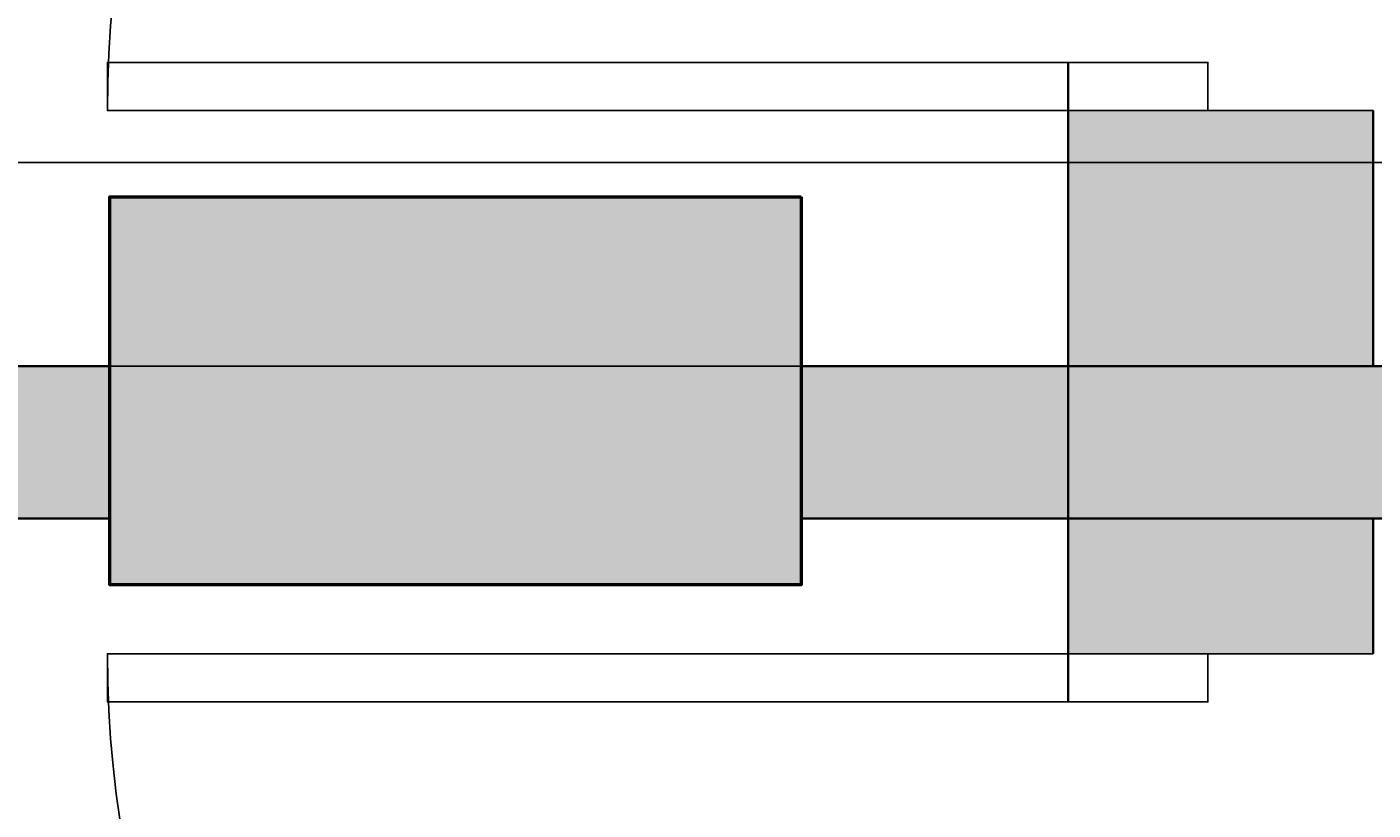
# Model space of a CAD drawing. Units: inches. Extents: x 1998 to 2588, y 1139 to 1977.
# Tile 8 of 134: x 2075 to 2115, y 1576 to 1599. Entities that reach past the tile are written whole.
import ezdxf

# ---------------------------------------------------------------- set-up
doc = ezdxf.new("R2010")
doc.units = ezdxf.units.IN
for name, color, linetype, lineweight in [('A-ANNO-DIMS', 2, 'Continuous', 18), ('A-COLS-PATT', 250, 'Continuous', 13), ('A-WALL-PATT', 252, 'Continuous', 13), ('COLUMN', 10, 'Continuous', 50), ('DOOR', 52, 'Continuous', 25), ('WALL', 200, 'Continuous', 35)]:
    doc.layers.add(name, color=color, linetype=linetype, lineweight=lineweight)
doc.styles.get("Standard").update_dxf_attribs({"font": 'arial.ttf'})
doc.dimstyles.get("Standard").update_dxf_attribs({"dimtxt": 0.18, "dimasz": 0.18, "dimexe": 0.18, "dimexo": 0.0625, "dimgap": 0.09, "dimtad": 0, "dimtih": 1, "dimtoh": 1, "dimdec": 4, "dimzin": 0, "dimdsep": 46, "dimtxsty": 'Standard', "dimcen": 0.09, "dimadec": 0, "dimazin": 0, "dimtfac": 1, "dimtdec": 4, "dimtofl": 0, "dimtmove": 0, "dimatfit": 3, "dimfxl": 1, "dimtolj": 1, "dimtzin": 0, "dimarcsym": 0})

# ---------------------------------------------------------------- blocks, each defined once
blk = doc.blocks.new('*U2')
for p, q in [((0, 0), (0, -6)), ((40, 0), (40, -6))]:
    blk.add_line(p, q)
blk.add_lwpolyline([(0, 0), (0, 40), (1.75, 40), (1.75, 0)], close=True)
blk.add_arc((0, 0), 40, 0, 90)
blk = doc.blocks.new('*D30')
at = {"layer": 'A-ANNO-DIMS', "color": 0, "lineweight": -2, "transparency": 16777216}
for p, q in [((2407.91, 1636.732), (1997.843, 1636.732)), ((1998.023, 1636.552), (1998.023, 1615.913)), ((1998.023, 1594.912), (1998.023, 1615.552)), ((2407.91, 1594.732), (1997.843, 1594.732))]:
    blk.add_line(p, q, dxfattribs=at)
at = {"layer": 'A-ANNO-DIMS', "color": 0, "transparency": 16777216}
for points in [[(1997.993, 1636.552), (1998.053, 1636.552), (1998.023, 1636.732)], [(1997.993, 1594.912), (1998.053, 1594.912), (1998.023, 1594.732)]]:
    blk.add_solid(points, dxfattribs=at)
at = {"layer": 'Defpoints', "color": 0, "transparency": 16777216}
for p in [(1998.023, 1636.732), (2407.973, 1636.732), (2407.973, 1594.732)]:
    blk.add_point(p, dxfattribs=at)
at = {"layer": 'A-ANNO-DIMS', "color": 0, "transparency": 16777216, "insert": (1998.023, 1615.732), "char_height": 0.18, "attachment_point": 5}
blk.add_mtext('\\A1;42', dxfattribs=at)
blk = doc.blocks.new('*D34')
at = {"layer": 'A-ANNO-DIMS', "color": 0, "lineweight": -2, "transparency": 16777216}
for p, q in [((2407.91, 1594.732), (1997.843, 1594.732)), ((1998.023, 1594.552), (1998.023, 1558.913)), ((1998.023, 1522.912), (1998.023, 1558.552)), ((2407.91, 1522.732), (1997.843, 1522.732))]:
    blk.add_line(p, q, dxfattribs=at)
at = {"layer": 'A-ANNO-DIMS', "color": 0, "transparency": 16777216}
for points in [[(1997.993, 1594.552), (1998.053, 1594.552), (1998.023, 1594.732)], [(1997.993, 1522.912), (1998.053, 1522.912), (1998.023, 1522.732)]]:
    blk.add_solid(points, dxfattribs=at)
at = {"layer": 'Defpoints', "color": 0, "transparency": 16777216}
for p in [(1998.023, 1594.732), (2407.973, 1594.732), (2407.973, 1522.732)]:
    blk.add_point(p, dxfattribs=at)
at = {"layer": 'A-ANNO-DIMS', "color": 0, "transparency": 16777216, "insert": (1998.023, 1558.732), "char_height": 0.18, "attachment_point": 5}
blk.add_mtext('\\A1;72', dxfattribs=at)
blk = doc.blocks.new('*D35')
at = {"layer": 'A-ANNO-DIMS', "color": 0, "lineweight": -2, "transparency": 16777216}
for p, q in [((2148.392, 1612.732), (1997.843, 1612.732)), ((1998.023, 1612.552), (1998.023, 1600.913)), ((1998.023, 1588.912), (1998.023, 1600.552)), ((2148.392, 1588.732), (1997.843, 1588.732))]:
    blk.add_line(p, q, dxfattribs=at)
at = {"layer": 'A-ANNO-DIMS', "color": 0, "transparency": 16777216}
for points in [[(1997.993, 1612.552), (1998.053, 1612.552), (1998.023, 1612.732)], [(1997.993, 1588.912), (1998.053, 1588.912), (1998.023, 1588.732)]]:
    blk.add_solid(points, dxfattribs=at)
at = {"layer": 'Defpoints', "color": 0, "transparency": 16777216}
for p in [(1998.023, 1612.732), (2148.455, 1612.732), (2148.455, 1588.732)]:
    blk.add_point(p, dxfattribs=at)
at = {"layer": 'A-ANNO-DIMS', "color": 0, "transparency": 16777216, "insert": (1998.023, 1600.732), "char_height": 0.18, "attachment_point": 5}
blk.add_mtext('\\A1;24', dxfattribs=at)

msp = doc.modelspace()

# ---------------------------------------------------------------- hatches: boundary and pattern name
at = {"layer": 'A-COLS-PATT'}
h = msp.add_hatch(color=256, dxfattribs=at)
h.dxf.hatch_style = 1
h.paths.add_polyline_path([(2099.4125, 1888.7324), (2087.9729, 1888.7324), (2087.9729, 1868.3278), (2099.4125, 1868.3278)])
h.paths.add_polyline_path([(2234.4125, 1888.7324), (2222.9729, 1888.7324), (2222.9729, 1868.3278), (2234.4125, 1868.3278)])
h.paths.add_polyline_path([(2341.4729, 1886.637), (2330.0332, 1886.637), (2330.0332, 1866.2324), (2341.4729, 1866.2324)])
h.paths.add_polyline_path([(2507.8006, 1882.7324), (2487.396, 1882.7324), (2487.396, 1871.2927), (2507.8006, 1871.2927)])
h.paths.add_polyline_path([(2510.9729, 1766.672), (2490.5682, 1766.672), (2490.5682, 1755.2324), (2510.9729, 1755.2324)])
h.paths.add_polyline_path([(2345.9729, 1759.7324), (2334.5332, 1759.7324), (2334.5332, 1739.3278), (2345.9729, 1739.3278)])
h.paths.add_polyline_path([(2234.4125, 1774.3318), (2222.9729, 1774.3318), (2222.9729, 1753.9272), (2234.4125, 1753.9272)])
h.paths.add_polyline_path([(2099.4125, 1775.637), (2087.9729, 1775.637), (2087.9729, 1755.2324), (2099.4125, 1755.2324)])
h.paths.add_polyline_path([(2098.0956, 1593.7241), (2077.691, 1593.7241), (2077.691, 1582.2845), (2098.0956, 1582.2845)])
h.paths.add_polyline_path([(2227.4729, 1604.637), (2216.0332, 1604.637), (2216.0332, 1584.2324), (2227.4729, 1584.2324)])
h.paths.add_polyline_path([(2345.9729, 1647.5211), (2334.5332, 1647.5211), (2334.5332, 1627.1165), (2345.9729, 1627.1165)])
h.paths.add_polyline_path([(2522.3775, 1641.2324), (2501.9729, 1641.2324), (2501.9729, 1629.7927), (2522.3775, 1629.7927)])
h.paths.add_polyline_path([(2522.3775, 1480.7324), (2501.9729, 1480.7324), (2501.9729, 1469.2927), (2522.3775, 1469.2927)])
h.paths.add_polyline_path([(2345.9729, 1488.5616), (2334.5332, 1488.5616), (2334.5332, 1468.1569), (2345.9729, 1468.1569)])
h.paths.add_polyline_path([(2234.4125, 1486.137), (2227.4729, 1486.137), (2227.4729, 1465.7324), (2234.4125, 1465.7324)])
h.paths.add_polyline_path([(2227.4729, 1486.137), (2222.9729, 1486.137), (2222.9729, 1465.7324), (2227.4729, 1465.7324)])
h.paths.add_polyline_path([(2108.3775, 1470.2324), (2087.9729, 1470.2324), (2087.9729, 1458.7927), (2108.3775, 1458.7927)])
h.paths.add_polyline_path([(2096.9729, 1365.5012), (2087.9729, 1365.5012), (2087.9729, 1345.0966), (2096.9729, 1345.0966)])
h.paths.add_polyline_path([(2087.9729, 1365.5012), (2085.5332, 1365.5012), (2085.5332, 1345.0966), (2087.9729, 1345.0966)])
h.paths.add_polyline_path([(2234.4125, 1285.137), (2222.9729, 1285.137), (2222.9729, 1264.7324), (2234.4125, 1264.7324)])
h.paths.add_polyline_path([(2345.9729, 1285.137), (2334.5332, 1285.137), (2334.5332, 1264.7324), (2345.9729, 1264.7324)])
h.paths.add_polyline_path([(2503.1458, 1240.172), (2482.7412, 1240.172), (2482.7412, 1228.7324), (2503.1458, 1228.7324)])
h.paths.add_polyline_path([(2510.9729, 1369.172), (2490.5682, 1369.172), (2490.5682, 1357.7324), (2510.9729, 1357.7324)])
at = {"layer": 'A-WALL-PATT'}
h = msp.add_hatch(color=256, dxfattribs=at)
h.dxf.hatch_style = 1
h.paths.add_polyline_path([(2222.9729, 1888.7324), (2099.4125, 1888.7324), (2099.4125, 1879.7324), (2222.9729, 1879.7324)])
h.paths.add_polyline_path([(2096.9729, 1868.3278), (2087.9729, 1868.3278), (2087.9729, 1775.637), (2096.9729, 1775.637)])
h.paths.add_polyline_path([(2227.4729, 1868.3278), (2222.9729, 1868.3278), (2222.9729, 1774.3318), (2227.4729, 1774.3318)])
h.paths.add_polyline_path([(2188.3019, 1759.7324), (2138.6074, 1759.7324), (2099.4125, 1759.7324), (2099.4125, 1755.2324), (2176.9729, 1755.2324), (2188.3019, 1755.2324)])
h.paths.add_polyline_path([(2087.9729, 1759.7324), (2059.4729, 1759.7324), (2059.4729, 1702.7324), (2087.9729, 1702.7324), (2087.9729, 1707.2324), (2063.9729, 1707.2324), (2063.9729, 1755.2324), (2087.9729, 1755.2324)])
h.paths.add_polyline_path([(2096.9729, 1755.2324), (2087.9729, 1755.2324), (2087.9729, 1707.2324), (2096.9729, 1707.2324)])
h.paths.add_polyline_path([(2187.0461, 1707.2324), (2105.9729, 1707.2324), (2096.9729, 1707.2324), (2087.9729, 1707.2324), (2087.9729, 1702.7324), (2105.9729, 1702.7324), (2114.9729, 1702.7324), (2187.0461, 1702.7324)])
h.paths.add_polyline_path([(2181.4729, 1719.2028), (2176.9729, 1719.2028), (2176.9729, 1707.2324), (2181.4729, 1707.2324)])
h.paths.add_polyline_path([(2216.0332, 1588.7324), (2114.9729, 1588.7324), (2105.9729, 1588.7324), (2105.9729, 1584.2324), (2216.0332, 1584.2324)])
h.paths.add_polyline_path([(2077.691, 1588.7324), (2061.4729, 1588.7324), (2061.4729, 1584.2324), (2077.691, 1584.2324)])
h.paths.add_polyline_path([(2105.9729, 1588.7324), (2098.0956, 1588.7324), (2098.0956, 1584.2324), (2105.9729, 1584.2324)])
h.paths.add_polyline_path([(2114.9729, 1596.2642), (2110.1012, 1596.2642), (2105.9729, 1596.2642), (2105.9729, 1588.7324), (2114.9729, 1588.7324)])
h.paths.add_polyline_path([(2114.9729, 1584.2324), (2105.9729, 1584.2324), (2105.9729, 1580.249), (2110.1012, 1580.249), (2114.9729, 1580.249)])
h.paths.add_polyline_path([(2114.9729, 1547.7716), (2110.1012, 1547.7716, -0.0318759), (2105.9729, 1548.035), (2105.9729, 1470.2324), (2108.3775, 1470.2324), (2108.3775, 1465.7324), (2186.2943, 1465.7324), (2186.2943, 1470.2324), (2114.9729, 1470.2324)])
h.paths.add_polyline_path([(2227.4729, 1584.2324), (2222.9729, 1584.2324), (2222.9729, 1486.137), (2227.4729, 1486.137)])
h.paths.add_polyline_path([(2295.4138, 1593.2324), (2227.4729, 1593.2324), (2227.4729, 1588.7324), (2295.4138, 1588.7324), (2295.4138, 1591.8729)])
h.paths.add_polyline_path([(2345.9729, 1627.1165), (2341.4729, 1627.1165), (2341.4729, 1593.2324), (2337.2869, 1593.2324), (2337.2869, 1591.8729), (2337.2869, 1588.7324), (2345.9729, 1588.7324)])
h.paths.add_polyline_path([(2291.9729, 1588.7324), (2287.4729, 1588.7324), (2287.4729, 1522.7324), (2291.9729, 1522.7324)])
h.paths.add_polyline_path([(2291.9729, 1522.7324), (2287.4729, 1522.7324), (2227.4729, 1522.7324), (2227.4729, 1518.2324), (2291.9729, 1518.2324)])
h.paths.add_polyline_path([(2295.7347, 1519.5919), (2295.7347, 1522.7324), (2291.9729, 1522.7324), (2291.9729, 1518.2324), (2295.7347, 1518.2324)])
h.paths.add_polyline_path([(2345.9729, 1522.7324), (2337.6078, 1522.7324), (2337.6078, 1519.5919), (2337.6078, 1518.2324), (2341.4729, 1518.2324), (2341.4729, 1488.5616), (2345.9729, 1488.5616)])
h.paths.add_polyline_path([(2345.9729, 1468.1569), (2341.4729, 1468.1569), (2341.4729, 1374.2324), (2227.4729, 1374.2324), (2227.4729, 1369.7324), (2345.9729, 1369.7324)])
h.paths.add_polyline_path([(2345.9729, 1369.7324), (2341.4729, 1369.7324), (2341.4729, 1362.2324), (2345.9729, 1362.2324)])
h.paths.add_polyline_path([(2345.9729, 1317.7324), (2345.9729, 1322.2324), (2341.4729, 1322.2324), (2341.4729, 1285.137), (2345.9729, 1285.137)], flags=17)
h.paths.add_polyline_path([(2356.2096, 1322.2324), (2345.9729, 1322.2324), (2345.9729, 1317.7324), (2356.2096, 1317.7324), (2356.2096, 1319.3088)], flags=17)
h.paths.add_polyline_path([(2393.9729, 1322.2324), (2375.6999, 1322.2324), (2375.6999, 1319.3088, -0.0202458), (2375.636, 1317.7324), (2393.9729, 1317.7324)], flags=17)
h.paths.add_polyline_path([(2398.4729, 1322.2324), (2393.9729, 1322.2324), (2393.9729, 1317.7324), (2393.9729, 1237.7324), (2345.9729, 1237.7324), (2345.9729, 1264.7324), (2341.4729, 1264.7324), (2341.4729, 1228.7324), (2393.9729, 1228.7324), (2482.7412, 1228.7324), (2482.7412, 1237.7324), (2398.4729, 1237.7324), (2398.4729, 1297.1029)])
h.paths.add_polyline_path([(2398.4729, 1362.2324), (2393.9729, 1362.2324), (2393.9729, 1357.7324), (2398.4729, 1357.7324)])
h.paths.add_polyline_path([(2345.9729, 1329.7549), (2341.4729, 1329.7549), (2341.4729, 1322.2324), (2345.9729, 1322.2324)])

# ---------------------------------------------------------------- linework, layer by layer
at = {"layer": 'COLUMN'}
msp.add_lwpolyline([(2098.0956, 1593.7241), (2098.0956, 1582.2845), (2077.691, 1582.2845), (2077.691, 1593.7241)], close=True, dxfattribs=at)
at = {"layer": 'WALL'}
for p, q in [((2105.9729, 1584.2324), (2105.9729, 1597.6851)), ((2114.9729, 1588.7324), (2114.9729, 1596.2642)), ((2077.691, 1588.7324), (2061.4729, 1588.7324)), ((2114.9729, 1588.7324), (2098.0956, 1588.7324)), ((2216.0332, 1588.7324), (2114.9729, 1588.7324)), ((2077.691, 1584.2324), (2061.4729, 1584.2324)), ((2105.9729, 1584.2324), (2098.0956, 1584.2324)), ((2227.4729, 1584.2324), (2105.9729, 1584.2324)), ((2105.9729, 1578.8281), (2105.9729, 1584.2324)), ((2114.9729, 1580.249), (2114.9729, 1584.2324))]:
    msp.add_line(p, q, dxfattribs=at)

# ---------------------------------------------------------------- block references
at = {"layer": 'DOOR', "yscale": 0.8119355758402486, "zscale": 0.8119355758402486}
for p, xscale, rotation in [((2110.1012, 1596.2642), 0.8119355758402486, 90.00000000000003), ((2110.1012, 1580.249), -0.8119355758402486, 90)]:
    msp.add_blockref('*U2', p, dxfattribs=dict(at, xscale=xscale, rotation=rotation))

# ---------------------------------------------------------------- dimensions: what is measured, and where the dimension line sits
at = {"layer": 'A-ANNO-DIMS'}
for base, p1, p2, picture, middle in [((1998.0229, 1636.7324), (2407.9729, 1594.7324), (2407.9729, 1636.7324), '*D30', (1998.0229, 1615.7324)), ((1998.0229, 1612.7324), (2148.4548, 1588.7324), (2148.4548, 1612.7324), '*D35', (1998.0229, 1600.7324)), ((1998.0229, 1594.7324), (2407.9729, 1522.7324), (2407.9729, 1594.7324), '*D34', (1998.0229, 1558.7324))]:
    dim = msp.add_linear_dim(base=base, p1=p1, p2=p2, angle=90, dimstyle='Standard', override={"dimdec": 0, "dimlfac": 1, "dimrnd": 0, "dimzin": 0, "dimdsep": 46, "dimlunit": 2}, dxfattribs=at)
    dim.commit()
    dim.dimension.update_dxf_attribs({"geometry": picture, "text_midpoint": middle})

doc.saveas('drawing.dxf')
